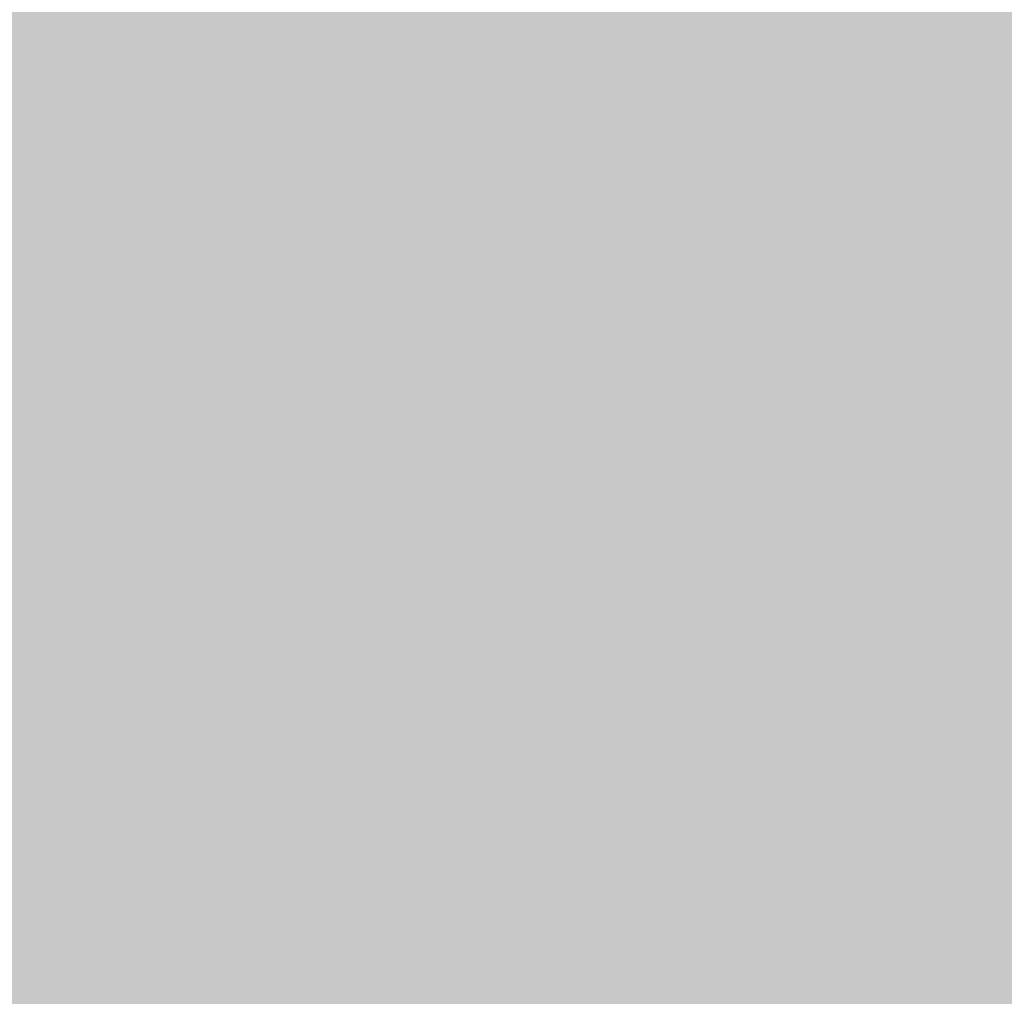
# Model space of a CAD drawing. Units: inches. Extents: x 2083 to 3317, y 1141 to 2115.
# Tile 162 of 256: x 3126.958245 to 3126.959398, y 1263.262504 to 1263.263648. Entities that reach past the tile are written whole.
import ezdxf

# ---------------------------------------------------------------- set-up
doc = ezdxf.new("R2010")
doc.units = ezdxf.units.IN
doc.layers.add('A-WALL-PATT', color=251, linetype='Continuous', lineweight=13, true_color=0x636466)

msp = doc.modelspace()

# ---------------------------------------------------------------- hatches: boundary and pattern name
at = {"layer": 'A-WALL-PATT'}
h = msp.add_hatch(color=256, dxfattribs=at)
h.dxf.hatch_style = 1
h.paths.add_polyline_path([(3126.9597832, 2020.7613601), (2748.9597832, 2020.7613601), (2604.9597832, 2020.7613601), (2226.9597832, 2020.7613601), (2226.9597832, 1702.7613601), (2466.9597832, 1702.7613601), (2466.9597832, 1582.7613601), (2418.9597832, 1582.7613601), (2418.9597832, 1477.7613601), (2226.9597832, 1477.7613601), (2226.9597832, 1263.2613601), (2544.9597832, 1263.2613601), (2544.9597832, 1411.7613601), (2604.9597832, 1411.7613601), (2685.9597832, 1411.7613601), (2685.9597832, 1420.7613601), (2604.9597832, 1420.7613601), (2604.9597832, 1573.7613601), (2604.9597832, 1702.7613601), (2604.9597832, 2011.7613601), (2748.9597832, 2011.7613601), (2748.9597832, 1702.7613601), (2862.9597832, 1702.7613601), (2862.9597832, 1621.7613601), (2871.9597832, 1621.7613601), (2871.9597832, 1702.7613601), (2883.9597832, 1702.7613601), (2883.9597832, 1706.9394595, -0.026459), (2883.9597832, 1711.7613601), (2757.9597832, 1711.7613601), (2757.9597832, 1807.7613601), (2787.9597832, 1807.7613601), (2787.9597832, 1812.2613601), (2757.9597832, 1812.2613601), (2757.9597832, 2011.7613601), (2877.9597832, 2011.7613601), (2877.9597832, 1812.2613601), (2847.9597832, 1812.2613601), (2847.9597832, 1807.7613601), (2889.8357425, 1807.7613601), (2889.8357425, 1812.2613601), (2882.4597832, 1812.2613601), (2882.4597832, 2011.7613601), (3117.9597832, 2011.7613601), (3117.9597832, 1812.2613601), (2937.8357425, 1812.2613601), (2937.8357425, 1807.7613601), (2995.7097832, 1807.7613601), (2995.7097832, 1796.1176655), (3000.2097832, 1796.1176655), (3000.2097832, 1807.7613601), (3117.9597832, 1807.7613601), (3117.9597832, 1711.7613601), (3000.2097832, 1711.7613601), (3000.2097832, 1760.1176655), (2998.5727047, 1760.1176655, -0.020711), (2995.7097832, 1760.1176655), (2995.7097832, 1711.7613601), (2931.9597832, 1711.7613601), (2931.9597832, 1702.7613601), (3126.9597832, 1702.7613601)])
h.paths.add_polyline_path([(2471.4597832, 2011.7613601), (2471.4597832, 1810.0113601), (2462.7169357, 1810.0113601), (2462.7169357, 1805.5113601), (2505.9597832, 1805.5113601), (2505.9597832, 1810.0113601), (2475.9597832, 1810.0113601), (2475.9597832, 2011.7613601), (2595.9597832, 2011.7613601), (2595.9597832, 1810.0113601), (2565.9597832, 1810.0113601), (2565.9597832, 1805.5113601), (2595.9597832, 1805.5113601), (2595.9597832, 1711.7613601), (2235.9597832, 1711.7613601), (2235.9597832, 1805.5113601), (2353.7097832, 1805.5113601), (2353.7097832, 1796.0541624), (2358.2097832, 1796.0541624), (2358.2097832, 1805.5113601), (2414.7169357, 1805.5113601), (2414.7169357, 1810.0113601), (2235.9597832, 1810.0113601), (2235.9597832, 2011.7613601)], flags=16)
h.paths.add_polyline_path([(2270.2047343, 1994.6100082), (2270.2047343, 1970.6100082), (2246.2047343, 1970.6100082), (2246.2047343, 1994.6100082)], flags=0)
edge = h.paths.add_edge_path(flags=0)
edge.add_ellipse((2332.027391, 1899.7981761), major_axis=(-3.0429938, 3.0429938), ratio=0.16825245, start_angle=-161.3321656, end_angle=-156.3071136, ccw=False)
edge.add_ellipse((2333.0820373, 1898.7435297), major_axis=(-1.0546463, 1.0546463), ratio=0.453532097, start_angle=-123.371019, end_angle=-94.1591066)
edge = h.paths.add_edge_path(flags=0)
edge.add_ellipse((2332.027391, 1968.8762897), major_axis=(3.0429938, 3.0429938), ratio=0.16825245, start_angle=18.6678344, end_angle=23.6928864)
edge.add_spline(control_points=[(2332.9255964, 1970.6911045), (2332.2267681, 1970.3360997), (2330.8937087, 1969.6589054), (2328.4130803, 1970.9321376), (2327.2039345, 1967.7487119), (2324.7095965, 1969.9555886), (2322.5328223, 1967.012354), (2320.0128462, 1971.2958124), (2317.6803077, 1968.1578449), (2316.0405263, 1967.1020468), (2315.4269045, 1966.8096022)], knot_values=[0, 0, 0, 0, 2.267059, 4.324559, 6.685584, 8.878641, 11.121502, 14.300359, 17.755284, 19.732645, 19.732645, 19.732645, 19.732645], degree=3, periodic=0)
edge.add_ellipse((2332.027391, 1968.8762897), major_axis=(3.0429938, 3.0429938), ratio=0.16825245, start_angle=18.6678344, end_angle=23.6928864, ccw=False)
edge.add_ellipse((2333.0820373, 1969.930936), major_axis=(1.0546463, 1.0546463), ratio=0.453532097, start_angle=56.628981, end_angle=85.8408934, ccw=False)
edge = h.paths.add_edge_path(flags=0)
edge.add_spline(control_points=[(2296.4282874, 1967.9879081), (2293.6278045, 1965.3363137), (2287.7036238, 1959.727094), (2299.7438601, 1949.9956993), (2294.5325909, 1935.6685275), (2290.5732281, 1920.6035119), (2293.3941244, 1909.9736911), (2296.1854073, 1904.9665431)], knot_values=[0.099185, 0.099185, 0.099185, 0.099185, 0.345301, 0.619822, 0.982653, 1.386093, 1.810555, 1.810555, 1.810555, 1.810555], degree=3, periodic=0)
edge.add_spline(control_points=[(2296.1854073, 1904.9665431), (2297.3835817, 1902.6193002), (2298.0009694, 1901.9493116), (2298.5529698, 1901.4681549)], knot_values=[0.006246, 0.006246, 0.006246, 0.006246, 0.055476, 0.055476, 0.055476, 0.055476], degree=3, periodic=0)
edge.add_spline(control_points=[(2298.5529698, 1901.4681549), (2297.2586121, 1900.9232238), (2295.2252939, 1900.2321257), (2293.0602287, 1900.6142053), (2292.1014227, 1900.788415), (2292.0895776, 1900.790568)], knot_values=[0.312835, 0.312835, 0.312835, 0.312835, 0.40178, 0.474987, 0.475903, 0.475903, 0.475903, 0.475903], degree=3, periodic=0)
edge.add_arc((2292.7936464, 1904.6641088), 3.9370079, 215.4208969, 259.6981795, ccw=False)
edge.add_spline(control_points=[(2289.5853139, 1902.3823039), (2289.4766524, 1902.5350874), (2289.3684805, 1902.6880353), (2289.2608648, 1902.8411699)], knot_values=[0.102872, 0.102872, 0.102872, 0.102872, 0.116896, 0.116896, 0.116896, 0.116896], degree=3, periodic=0)
edge.add_spline(control_points=[(2289.2608648, 1902.8411699), (2288.6866042, 1902.5501922), (2287.6400477, 1902.0199025), (2285.8813368, 1901.8739536), (2283.8529717, 1901.5043521), (2281.7199871, 1899.7105375), (2278.4669913, 1899.492942), (2276.1571361, 1901.8832022), (2272.2589526, 1899.8040711), (2267.7776054, 1901.8431828), (2262.2438819, 1900.1840326), (2257.414927, 1901.7820606), (2254.318374, 1900.7261196), (2253.1782849, 1900.3373431)], knot_values=[0, 0, 0, 0, 1.907977, 3.477176, 5.261074, 7.972851, 11.680248, 13.717921, 16.939592, 22.789562, 27.502503, 33.595215, 37.145618, 37.145618, 37.145618, 37.145618], degree=3, periodic=0)
edge.add_line((2253.1782849, 1900.3373431), (2250.2442397, 1902.8411699))
edge.add_line((2250.2442397, 1902.8411699), (2250.2442397, 1965.8332959))
edge.add_line((2250.2442397, 1965.8332959), (2253.1782849, 1968.3371226))
edge.add_spline(control_points=[(2253.1782849, 1968.3371226), (2254.318374, 1967.9483462), (2257.414927, 1966.8924051), (2262.2438819, 1968.4904332), (2267.7776054, 1966.8312829), (2271.5267301, 1968.5372172), (2273.8759143, 1967.8282895), (2274.2067012, 1967.7276424)], knot_values=[0, 0, 0, 0, 0.09018, 0.244935, 0.364644, 0.513233, 0.537855, 0.537855, 0.537855, 0.537855], degree=3, periodic=0)
edge.add_arc((2274.3528869, 1963.7933495), 3.9370079, 72.0511336, 92.1279492, ccw=False)
edge.add_arc((2281.2969331, 1985.2300027), 18.5962982, 252.05113361, 288.56572166)
edge.add_arc((2292.3167172, 1956.0288805), 12.6460805, 71.02678788, 113.77821843, ccw=False)
edge = h.paths.add_edge_path(flags=0)
edge.add_spline(control_points=[(2274.8994147, 1951.8561946), (2275.066156, 1951.6165924), (2275.2326866, 1951.3765878), (2275.3979871, 1951.1358545)], knot_values=[1.409916, 1.409916, 1.409916, 1.409916, 1.43159, 1.43159, 1.43159, 1.43159], degree=3, periodic=0)
edge.add_spline(control_points=[(2275.3979871, 1951.1358545), (2275.7921055, 1950.5618854), (2276.1792311, 1949.9837745), (2276.5455462, 1949.3971029)], knot_values=[1.358238, 1.358238, 1.358238, 1.358238, 1.409916, 1.409916, 1.409916, 1.409916], degree=3, periodic=0)
edge.add_line((2276.5455462, 1949.3971029), (2277.437289, 1947.8621847))
edge.add_spline(control_points=[(2277.437289, 1947.8621847), (2276.3038341, 1945.6731147), (2274.6396979, 1942.4268817), (2274.631615, 1938.0938998), (2272.7991237, 1930.8515498), (2274.3564261, 1943.8970461), (2275.9476814, 1947.9233558), (2276.5455462, 1949.3971029)], knot_values=[0.005632, 0.005632, 0.005632, 0.005632, 0.186014, 0.266002, 0.357087, 0.59639, 0.739732, 0.739732, 0.739732, 0.739732], degree=3, periodic=0)
edge.add_spline(control_points=[(2276.5455462, 1949.3971029), (2276.1792311, 1949.9837745), (2275.7921055, 1950.5618854), (2275.3979871, 1951.1358545)], knot_values=[1.358238, 1.358238, 1.358238, 1.358238, 1.409916, 1.409916, 1.409916, 1.409916], degree=3, periodic=0)
edge.add_spline(control_points=[(2275.3979871, 1951.1358545), (2274.9425002, 1950.0804523), (2274.2077604, 1948.0252718), (2273.9346018, 1944.8514774), (2272.4685341, 1937.6274891), (2273.4662155, 1945.6964663), (2274.7006154, 1951.0594725), (2274.8994147, 1951.8561946)], knot_values=[0.104364, 0.104364, 0.104364, 0.104364, 0.189636, 0.269624, 0.36071, 0.600013, 0.644622, 0.644622, 0.644622, 0.644622], degree=3, periodic=0)
h.paths.add_polyline_path([(2269.1675139, 1963.1275729, -0.357527), (2268.170633, 1960.9763695, -0.092561), (2268.170633, 1939.4363249, -0.357527), (2269.1675139, 1937.2851215, -0.357527), (2267.0163105, 1938.2820024, -0.164785), (2254.6855813, 1938.2820024, -0.357527), (2252.5343779, 1937.2851215, -0.357527), (2253.5312587, 1939.4363249, -0.092561), (2253.5312587, 1960.9763695, -0.357527), (2252.5343779, 1963.1275729, -0.357527), (2254.6855813, 1962.130692, -0.164785), (2267.0163105, 1962.130692, -0.357527)], flags=0)
h.paths.add_polyline_path([(2248.8740679, 1967.8017998), (2248.8740679, 1957.0277095), (2249.4577833, 1957.0277095), (2249.4577833, 1911.6467562), (2248.8740679, 1911.6467562), (2248.8740679, 1900.8726659), (2246.5118632, 1900.8726659, 0.197327), (2244.1496584, 1902.4568734), (2244.1496584, 1966.2175923, 0.197327), (2246.5118632, 1967.8017998)], flags=0)
h.paths.add_polyline_path([(2269.1675139, 1931.3893442, -0.357527), (2268.170633, 1929.2381408, -0.092561), (2268.170633, 1907.6980962, -0.357527), (2269.1675139, 1905.5468928, -0.357527), (2267.0163105, 1906.5437737, -0.164785), (2254.6855813, 1906.5437737, -0.357527), (2252.5343779, 1905.5468928, -0.357527), (2253.5312587, 1907.6980962, -0.092561), (2253.5312587, 1929.2381408, -0.357527), (2252.5343779, 1931.3893442, -0.357527), (2254.6855813, 1930.3924634, -0.164785), (2267.0163105, 1930.3924634, -0.357527)], flags=0)
edge = h.paths.add_edge_path(flags=0)
edge.add_spline(control_points=[(2276.1968578, 1906.7237016), (2276.1681442, 1909.0289278), (2276.1140492, 1913.371852), (2270.5984171, 1924.9249783), (2273.9051746, 1919.0127787), (2275.9217115, 1916.2620626), (2275.4745699, 1912.4021495), (2277.2578735, 1910.3806206), (2276.6960436, 1908.2250358), (2276.6462176, 1906.8130226), (2276.6178249, 1906.0084068)], knot_values=[0, 0, 0, 0, 8.61026, 16.221274, 18.843057, 23.804898, 27.440828, 29.356102, 31.203478, 33.650687, 33.650687, 33.650687, 33.650687], degree=3, periodic=0)
edge.add_spline(control_points=[(2276.6178249, 1906.0084068), (2276.6233131, 1905.6241436), (2276.4977381, 1904.6286608), (2275.4417789, 1903.8547251), (2274.9373144, 1903.0804497), (2274.8590804, 1902.8411699)], knot_values=[0.156488, 0.156488, 0.156488, 0.156488, 0.184398, 0.231376, 0.250598, 0.250598, 0.250598, 0.250598], degree=3, periodic=0)
edge.add_line((2274.8590804, 1902.8411699), (2276.50598, 1902.8411699))
edge.add_spline(control_points=[(2276.50598, 1902.8411699), (2276.7883084, 1903.0849395), (2277.6650711, 1904.1251958), (2278.2495378, 1904.340738), (2277.6538719, 1908.5273866), (2278.15567, 1906.2278078), (2278.100464, 1905.2859484), (2278.8466748, 1904.0690054), (2277.8567853, 1903.4149482), (2277.8741909, 1902.9910497), (2277.9035616, 1902.8411699)], knot_values=[0.059574, 0.059574, 0.059574, 0.059574, 0.080753, 0.103741, 0.16972, 0.176036, 0.207137, 0.240474, 0.262341, 0.27366, 0.27366, 0.27366, 0.27366], degree=3, periodic=0)
edge.add_line((2277.9035616, 1902.8411699), (2280.0298255, 1902.8411699))
edge.add_spline(control_points=[(2280.0298255, 1902.8411699), (2279.8882214, 1903.088398), (2279.4992571, 1903.9815512), (2280.1522839, 1905.9393491), (2278.103615, 1909.6577572), (2279.7623946, 1907.185285), (2280.3279002, 1904.8748608), (2280.4851086, 1903.4895904), (2281.4632687, 1903.2494323), (2281.7583431, 1902.9364967), (2281.8340361, 1902.8411699)], knot_values=[0.013856, 0.013856, 0.013856, 0.013856, 0.034874, 0.088867, 0.107879, 0.126738, 0.158714, 0.193757, 0.217487, 0.226722, 0.226722, 0.226722, 0.226722], degree=3, periodic=0)
edge.add_spline(control_points=[(2281.8340361, 1902.8411699), (2281.7875348, 1902.8267029), (2281.6470224, 1902.7829881), (2281.3955272, 1902.85949), (2281.088077, 1902.9852418), (2280.7206826, 1903.060902), (2280.3334513, 1903.0257257), (2280.1247668, 1902.898879), (2280.0298255, 1902.8411699)], knot_values=[0, 0, 0, 0, 0.14413, 0.435517, 0.749276, 1.153046, 1.548371, 1.878348, 1.878348, 1.878348, 1.878348], degree=3, periodic=0)
edge.add_line((2280.0298255, 1902.8411699), (2277.9035616, 1902.8411699))
edge.add_spline(control_points=[(2277.9035616, 1902.8411699), (2277.892855, 1902.7958553), (2277.865396, 1902.6796374), (2277.6074793, 1902.6874828), (2277.2740503, 1902.8006999), (2276.8379209, 1902.6197745), (2276.5838074, 1902.7892611), (2276.50598, 1902.8411699)], knot_values=[0, 0, 0, 0, 0.127189, 0.326199, 0.628009, 1.24357, 1.515331, 1.515331, 1.515331, 1.515331], degree=3, periodic=0)
edge.add_line((2276.50598, 1902.8411699), (2274.8590804, 1902.8411699))
edge.add_spline(control_points=[(2274.8590804, 1902.8411699), (2274.8144367, 1902.8985868), (2274.7251297, 1903.013446), (2274.4934765, 1903.1189684), (2274.2442854, 1902.9605386), (2273.9371207, 1903.1849416), (2273.6140395, 1902.9831428), (2273.4083164, 1902.8830449), (2273.322254, 1902.8411699)], knot_values=[0, 0, 0, 0, 0.21843, 0.436957, 0.687977, 0.990379, 1.398396, 1.69185, 1.69185, 1.69185, 1.69185], degree=3, periodic=0)
edge.add_spline(control_points=[(2273.322254, 1902.8411699), (2273.6167403, 1903.445692), (2274.2739977, 1904.5382529), (2276.0272387, 1904.5737017), (2276.2069634, 1906.5836372), (2276.1968578, 1906.7237016)], knot_values=[0.012227, 0.012227, 0.012227, 0.012227, 0.059472, 0.106218, 0.134458, 0.134458, 0.134458, 0.134458], degree=3, periodic=0)
h.paths.add_polyline_path([(2270.7760538, 1897.7898284), (2270.7760538, 1873.7898284), (2246.7760538, 1873.7898284), (2246.7760538, 1897.7898284)], flags=0)
h.paths.add_polyline_path([(2353.7097832, 1760.0050593), (2353.7097832, 1760.0541624), (2358.2097832, 1760.0541624, -0.033729)], flags=0)
h.paths.add_polyline_path([(2321.8191188, 1737.5291862), (2341.9953271, 1737.5291862, -0.414214), (2343.2032727, 1736.3212406), (2343.2032727, 1721.0205964, -0.414214), (2341.9953271, 1719.8126508), (2321.8191188, 1719.8126508, -0.414214), (2320.6111732, 1721.0205964), (2320.6111732, 1736.3212406, -0.414214)], flags=0)
h.paths.add_polyline_path([(2324.2350099, 1736.3212406), (2339.5794359, 1736.3212406, -0.414214), (2341.9953271, 1733.9053494), (2341.9953271, 1725.4497302, -0.414214), (2339.5794359, 1723.033839), (2333.6805885, 1723.033839), (2333.8453172, 1722.0454666, -0.870646), (2335.4253988, 1721.8258934, -0.767327), (2333.922694, 1721.4232449), (2331.2910241, 1721.4232449, -0.767327), (2329.7883193, 1721.8258934, -0.870646), (2331.3684009, 1722.0454666), (2331.5331296, 1723.033839), (2324.2350099, 1723.033839, -0.414214), (2321.8191188, 1725.4497302), (2321.8191188, 1733.9053494, -0.414214)], flags=0)
h.paths.add_polyline_path([(2570.4837892, 1928.6154443), (2589.6837892, 1928.6154443), (2590.1688286, 1928.6154443), (2590.1688286, 1904.9933971), (2570.4837892, 1904.9933971)], flags=0)
h.paths.add_polyline_path([(2574.4473242, 1927.2638215, -1), (2572.8288357, 1927.2638215, -1)], flags=0)
h.paths.add_polyline_path([(2573.0898665, 1926.9408768), (2573.925032, 1927.7760423), (2574.1477428, 1927.5533315), (2573.3125773, 1926.718166)], flags=0)
h.paths.add_polyline_path([(2578.7790648, 1919.7296175, -1), (2571.5916632, 1919.7296175, -1)], flags=0)
h.paths.add_polyline_path([(2578.385364, 1919.7296175, -1), (2571.985364, 1919.7296175, -1)], flags=0)
h.paths.add_polyline_path([(2331.5957638, 1729.4762156, -1), (2333.6179542, 1729.4762156, -1)], flags=0)
h.paths.add_polyline_path([(2578.0342282, 1927.2638215, -1), (2576.4157396, 1927.2638215, -1)], flags=0)
h.paths.add_polyline_path([(2576.6888513, 1927.5310886), (2576.9115621, 1927.7537993), (2577.7467276, 1926.9186339), (2577.5240168, 1926.6959231)], flags=0)
h.paths.add_polyline_path([(2578.1390648, 1909.8595388, -1), (2572.2316632, 1909.8595388, -1)], flags=0)
h.paths.add_polyline_path([(2577.745364, 1909.8595388, -1), (2572.625364, 1909.8595388, -1)], flags=0)
h.paths.add_polyline_path([(2583.7977179, 1927.2638215, -1), (2582.1792294, 1927.2638215, -1)], flags=0)
h.paths.add_polyline_path([(2582.7186487, 1927.7537993), (2583.5538142, 1926.9186339), (2583.3311034, 1926.6959231), (2582.4959379, 1927.5310886)], flags=0)
h.paths.add_polyline_path([(2582.4959379, 1927.5310886), (2582.7186487, 1927.7537993), (2583.5538142, 1926.9186339), (2583.3311034, 1926.6959231)], flags=0)
h.paths.add_polyline_path([(2587.7390648, 1920.5296175, -1), (2581.8316632, 1920.5296175, -1)], flags=0)
h.paths.add_polyline_path([(2587.345364, 1920.5296175, -1), (2582.225364, 1920.5296175, -1)], flags=0)
h.paths.add_polyline_path([(2587.3846219, 1927.2638215, -1), (2585.7661333, 1927.2638215, -1)], flags=0)
h.paths.add_polyline_path([(2586.0819925, 1926.9802469), (2586.917158, 1927.8154124), (2587.1398688, 1927.5927016), (2586.3047033, 1926.7575361)], flags=0)
h.paths.add_polyline_path([(2588.3790648, 1910.6595388, -1), (2581.1916632, 1910.6595388, -1)], flags=0)
h.paths.add_polyline_path([(2587.985364, 1910.6595388, -1), (2581.585364, 1910.6595388, -1)], flags=0)
h.paths.add_polyline_path([(2417.1677288, 1729.4778955), (2437.3439372, 1729.4778955, -0.414214), (2438.5518828, 1728.2699499), (2438.5518828, 1712.9693057, -0.414214), (2437.3439372, 1711.7613601), (2417.1677288, 1711.7613601, -0.414214), (2415.9597832, 1712.9693057), (2415.9597832, 1728.2699499, -0.414214)], flags=0)
h.paths.add_polyline_path([(2419.58362, 1728.2699499), (2434.928046, 1728.2699499, -0.414214), (2437.3439372, 1725.8540587), (2437.3439372, 1717.3984395, -0.414214), (2434.928046, 1714.9825483), (2429.0291985, 1714.9825483), (2429.1939273, 1713.9941758, -0.870646), (2430.7740089, 1713.7746027, -0.767327), (2429.2713041, 1713.3719542), (2426.6396342, 1713.3719542, -0.767327), (2425.1369294, 1713.7746027, -0.870646), (2426.717011, 1713.9941758), (2426.8817397, 1714.9825483), (2419.58362, 1714.9825483, -0.414214), (2417.1677288, 1717.3984395), (2417.1677288, 1725.8540587, -0.414214)], flags=0)
h.paths.add_polyline_path([(2419.58362, 1728.2699499), (2434.928046, 1728.2699499, -0.414214), (2437.3439372, 1725.8540587), (2437.3439372, 1717.3984395, -0.414214), (2434.928046, 1714.9825483), (2429.0291985, 1714.9825483), (2428.3581177, 1719.0090337), (2427.5528206, 1719.0090337), (2426.8817397, 1714.9825483), (2419.58362, 1714.9825483, -0.414214), (2417.1677288, 1717.3984395), (2417.1677288, 1725.8540587, -0.414214)], flags=0)
h.paths.add_polyline_path([(2426.9443739, 1721.4249248, -1), (2428.9665643, 1721.4249248, -1)], flags=0)
h.paths.add_polyline_path([(2475.9597832, 1702.7613601), (2595.9597832, 1702.7613601), (2595.9597832, 1582.7613601), (2475.9597832, 1582.7613601)], flags=16)
h.paths.add_polyline_path([(2427.9597832, 1573.7613601), (2595.9597832, 1573.7613601), (2595.9597832, 1468.7613601), (2595.9597832, 1420.7613601), (2384.4597832, 1420.7613601), (2384.4597832, 1468.7613601), (2427.9597832, 1468.7613601)], flags=16)
h.paths.add_polyline_path([(2379.9597832, 1468.7613601), (2379.9597832, 1420.7613601), (2235.9597832, 1420.7613601), (2235.9597832, 1468.7613601)], flags=16)
h.paths.add_polyline_path([(2317.8159962, 1466.695767), (2337.9922045, 1466.695767, -0.414214), (2339.2001501, 1465.4878214), (2339.2001501, 1450.1871771, -0.414214), (2337.9922045, 1448.9792315), (2317.8159962, 1448.9792315, -0.414214), (2316.6080506, 1450.1871771), (2316.6080506, 1465.4878214, -0.414214)], flags=0)
h.paths.add_polyline_path([(2320.2318874, 1465.4878214), (2335.5763133, 1465.4878214, -0.414214), (2337.9922045, 1463.0719302), (2337.9922045, 1454.616311, -0.414214), (2335.5763133, 1452.2004198), (2329.6774659, 1452.2004198), (2329.8421946, 1451.2120473, -0.870646), (2331.4222762, 1450.9924742, -0.767327), (2329.9195714, 1450.5898257), (2327.2879015, 1450.5898257, -0.767327), (2325.7851967, 1450.9924742, -0.870646), (2327.3652783, 1451.2120473), (2327.530007, 1452.2004198), (2320.2318874, 1452.2004198, -0.414214), (2317.8159962, 1454.616311), (2317.8159962, 1463.0719302, -0.414214)], flags=0)
h.paths.add_polyline_path([(2320.2318874, 1465.4878214), (2335.5763133, 1465.4878214, -0.414214), (2337.9922045, 1463.0719302), (2337.9922045, 1454.616311, -0.414214), (2335.5763133, 1452.2004198), (2329.6774659, 1452.2004198), (2329.006385, 1456.2269051), (2328.2010879, 1456.2269051), (2327.530007, 1452.2004198), (2320.2318874, 1452.2004198, -0.414214), (2317.8159962, 1454.616311), (2317.8159962, 1463.0719302, -0.414214)], flags=0)
h.paths.add_polyline_path([(2327.5926413, 1458.6427963, -1), (2329.6148317, 1458.6427963, -1)], flags=0)
h.paths.add_polyline_path([(2244.4117436, 1433.3404531), (2241.9209449, 1433.3404531, -0.414214), (2240.0178562, 1435.2435418), (2240.0178562, 1440.9528078, -0.414211), (2241.920925, 1442.8558965), (2244.4117436, 1442.8558965, -1.976472)], flags=0)
h.paths.add_polyline_path([(2245.3568884, 1434.3975358, -0.414214), (2245.3568884, 1441.7988138, -2.144098)], flags=0)
h.paths.add_polyline_path([(2535.9597832, 1416.2613601), (2535.9597832, 1272.2613601), (2235.9597832, 1272.2613601), (2235.9597832, 1416.2613601)], flags=16)
h.paths.add_polyline_path([(2260.1195614, 1384.2928413), (2260.1195614, 1362.0386487), (2237.8653688, 1362.0386487), (2237.8653688, 1384.2928413)], flags=0)
edge = h.paths.add_edge_path(flags=0)
edge.add_line((2318.2518466, 1362.0932983), (2318.1457968, 1362.0009726))
edge.add_ellipse((2317.4451158, 1360.4310442), major_axis=(2.8216404, 2.8216404), ratio=0.16825245, start_angle=18.6678344, end_angle=20.9481273, ccw=False)
edge.add_ellipse((2318.4230451, 1361.4089735), major_axis=(0.9779293, 0.9779293), ratio=0.453532097, start_angle=56.628981, end_angle=70.2262012, ccw=False)
edge = h.paths.add_edge_path(flags=0)
edge.add_line((2319.1073699, 1295.5710784), (2319.0150442, 1295.6771282))
edge.add_ellipse((2317.4451158, 1296.3778091), major_axis=(-2.8216404, 2.8216404), ratio=0.16825245, start_angle=-161.3321656, end_angle=-159.0518727, ccw=False)
edge.add_ellipse((2318.4230451, 1295.3998798), major_axis=(-0.9779293, 0.9779293), ratio=0.453532097, start_angle=-123.371019, end_angle=-109.7737988)
edge = h.paths.add_edge_path(flags=0)
edge.add_spline(control_points=[(2284.2103489, 1301.1702189), (2284.5806878, 1300.444719), (2284.8911891, 1299.8920243), (2285.159553, 1299.4610182)], knot_values=[0.039066, 0.039066, 0.039066, 0.039066, 0.055476, 0.055476, 0.055476, 0.055476], degree=3, periodic=0)
edge.add_line((2285.159553, 1299.4610182), (2284.2103489, 1301.1702189))
edge = h.paths.add_edge_path(flags=0)
edge.add_line((2280.4124579, 1297.2980125), (2283.3699905, 1297.0361216))
edge.add_line((2283.3699905, 1297.0361216), (2286.4056902, 1297.9263104))
edge.add_spline(control_points=[(2286.4056902, 1297.9263104), (2285.305487, 1297.4631193), (2284.3447774, 1297.1291508), (2283.3699905, 1297.0361216)], knot_values=[0.394369, 0.394369, 0.394369, 0.394369, 0.475903, 0.475903, 0.475903, 0.475903], degree=3, periodic=0)
edge.add_spline(control_points=[(2283.3699905, 1297.0361216), (2283.2813895, 1297.027666), (2282.316289, 1296.9573356), (2281.3125019, 1297.1344787), (2280.4234414, 1297.2960161), (2280.4124579, 1297.2980125)], knot_values=[0.312835, 0.312835, 0.312835, 0.312835, 0.320246, 0.393453, 0.394369, 0.394369, 0.394369, 0.394369], degree=3, periodic=0)
edge = h.paths.add_edge_path(flags=0)
edge.add_line((2284.4355615, 1359.6072854), (2280.4462909, 1355.328047))
edge.add_line((2280.4462909, 1355.328047), (2279.5799868, 1351.0177544))
edge.add_line((2279.5799868, 1351.0177544), (2282.4129737, 1346.5804327))
edge.add_spline(control_points=[(2282.4129737, 1346.5804327), (2283.1533308, 1345.5892358), (2284.2528957, 1344.0288973), (2284.801037, 1342.3871671), (2284.9351625, 1341.8055443)], knot_values=[1.240098, 1.240098, 1.240098, 1.240098, 1.332892, 1.382712, 1.382712, 1.382712, 1.382712], degree=3, periodic=0)
edge.add_spline(control_points=[(2284.9351625, 1341.8055443), (2285.3191079, 1340.1406002), (2285.2330291, 1338.4092041), (2284.9099384, 1336.6541222)], knot_values=[1.097484, 1.097484, 1.097484, 1.097484, 1.240098, 1.240098, 1.240098, 1.240098], degree=3, periodic=0)
edge.add_spline(control_points=[(2284.9099384, 1336.6541222), (2284.5868478, 1334.8990403), (2284.0267453, 1333.1202725), (2283.4626437, 1331.3605849)], knot_values=[0.95487, 0.95487, 0.95487, 0.95487, 1.097484, 1.097484, 1.097484, 1.097484], degree=3, periodic=0)
edge.add_line((2283.4626437, 1331.3605849), (2281.8903759, 1326.153357))
edge.add_line((2281.8903759, 1326.153357), (2280.7562592, 1321.0560888))
edge.add_line((2280.7562592, 1321.0560888), (2280.2992048, 1316.0019772))
edge.add_line((2280.2992048, 1316.0019772), (2280.7159327, 1310.9500678))
edge.add_line((2280.7159327, 1310.9500678), (2282.0280939, 1305.9721367))
edge.add_line((2282.0280939, 1305.9721367), (2284.2103489, 1301.1702189))
edge.add_spline(control_points=[(2284.2103489, 1301.1702189), (2283.3407305, 1302.7301854), (2282.6119044, 1304.3364933), (2282.0280939, 1305.9721367)], knot_values=[0.099185, 0.099185, 0.099185, 0.099185, 0.241799, 0.241799, 0.241799, 0.241799], degree=3, periodic=0)
edge.add_spline(control_points=[(2282.0280939, 1305.9721367), (2281.4442835, 1307.6077801), (2281.0054886, 1309.2727591), (2280.7159327, 1310.9500678)], knot_values=[0.241799, 0.241799, 0.241799, 0.241799, 0.384413, 0.384413, 0.384413, 0.384413], degree=3, periodic=0)
edge.add_spline(control_points=[(2280.7159327, 1310.9500678), (2280.4332411, 1312.5876134), (2280.2893863, 1314.2769594), (2280.2988938, 1315.9620324), (2280.2992048, 1316.0019772)], knot_values=[0.384413, 0.384413, 0.384413, 0.384413, 0.523647, 0.527028, 0.527028, 0.527028, 0.527028], degree=3, periodic=0)
edge.add_spline(control_points=[(2280.2992048, 1316.0019772), (2280.3123257, 1317.6869552), (2280.4778706, 1319.3679256), (2280.7562592, 1321.0560888)], knot_values=[0.527028, 0.527028, 0.527028, 0.527028, 0.669642, 0.669642, 0.669642, 0.669642], degree=3, periodic=0)
edge.add_spline(control_points=[(2280.7562592, 1321.0560888), (2281.0346478, 1322.7442519), (2281.4258801, 1324.4396079), (2281.8903759, 1326.153357)], knot_values=[0.669642, 0.669642, 0.669642, 0.669642, 0.812256, 0.812256, 0.812256, 0.812256], degree=3, periodic=0)
edge.add_spline(control_points=[(2281.8903759, 1326.153357), (2282.2643834, 1327.5332507), (2282.7878702, 1329.2618097), (2283.352751, 1331.0177803), (2283.4626437, 1331.3605849)], knot_values=[0.812256, 0.812256, 0.812256, 0.812256, 0.927087, 0.95487, 0.95487, 0.95487, 0.95487], degree=3, periodic=0)
edge.add_line((2283.4626437, 1331.3605849), (2284.9099384, 1336.6541222))
edge.add_line((2284.9099384, 1336.6541222), (2284.9351625, 1341.8055443))
edge.add_line((2284.9351625, 1341.8055443), (2282.4129737, 1346.5804327))
edge.add_spline(control_points=[(2282.4129737, 1346.5804327), (2281.2751273, 1348.1037918), (2280.0784467, 1349.5703178), (2279.5799868, 1351.0177544)], knot_values=[1.382712, 1.382712, 1.382712, 1.382712, 1.525326, 1.525326, 1.525326, 1.525326], degree=3, periodic=0)
edge.add_spline(control_points=[(2279.5799868, 1351.0177544), (2279.4432818, 1351.4147209), (2279.1363124, 1352.856922), (2279.7351897, 1354.2903851), (2280.4462909, 1355.328047)], knot_values=[1.525326, 1.525326, 1.525326, 1.525326, 1.564439, 1.667941, 1.667941, 1.667941, 1.667941], degree=3, periodic=0)
edge.add_spline(control_points=[(2280.4462909, 1355.328047), (2281.4261132, 1356.7578354), (2282.9308373, 1358.1825604), (2284.4355615, 1359.6072854)], knot_values=[1.667941, 1.667941, 1.667941, 1.667941, 1.810555, 1.810555, 1.810555, 1.810555], degree=3, periodic=0)
edge.add_arc((2280.6230749, 1348.518181), 11.7261796, 71.02678788, 113.77821843)
edge.add_arc((2270.4048917, 1375.5951559), 17.2435667, 252.05113361, 288.56572166, ccw=False)
edge.add_arc((2263.9659692, 1355.7178471), 3.6506221, 72.0511336, 92.1279492)
edge.add_arc((2263.9659692, 1355.7178471), 3.6506221, 92.1279492, 177.98513)
edge.add_spline(control_points=[(2260.3176041, 1355.8461989), (2260.2604169, 1354.2206683), (2260.551278, 1350.1865469), (2262.9993445, 1346.7662507), (2264.4727415, 1344.6490245)], knot_values=[1.43159, 1.43159, 1.43159, 1.43159, 1.564144, 1.770695, 1.770695, 1.770695, 1.770695], degree=3, periodic=0)
edge.add_line((2264.4727415, 1344.6490245), (2264.9355904, 1343.9825301))
edge.add_spline(control_points=[(2263.8010444, 1340.2481052), (2263.8432379, 1340.5140884), (2264.0672444, 1341.7564652), (2264.5126928, 1343.0024532), (2264.9350468, 1343.9810834)], knot_values=[0.53657, 0.53657, 0.53657, 0.53657, 0.559349, 0.644622, 0.644622, 0.644622, 0.644622], degree=3, periodic=0)
edge.add_spline(control_points=[(2264.9350468, 1343.9810834), (2265.1177715, 1343.7149747), (2265.2988751, 1343.4479058), (2265.4767562, 1343.1793646)], knot_values=[1.384077, 1.384077, 1.384077, 1.384077, 1.409916, 1.409916, 1.409916, 1.409916], degree=3, periodic=0)
edge.add_spline(control_points=[(2265.4767562, 1343.1793646), (2265.6546373, 1342.9108234), (2265.8292958, 1342.64081), (2265.9991301, 1342.368812)], knot_values=[1.358238, 1.358238, 1.358238, 1.358238, 1.384077, 1.384077, 1.384077, 1.384077], degree=3, periodic=0)
edge.add_line((2265.9991301, 1342.368812), (2266.8260057, 1340.9455468))
edge.add_spline(control_points=[(2266.8260057, 1340.9455468), (2268.894401, 1337.0896912), (2271.3981727, 1325.8430009), (2270.5161644, 1310.5685568), (2275.9193759, 1301.860609), (2277.7895113, 1299.1994495)], knot_values=[0.116896, 0.116896, 0.116896, 0.116896, 0.472987, 1.050969, 1.313793, 1.313793, 1.313793, 1.313793], degree=3, periodic=0)
edge.add_spline(control_points=[(2277.7895113, 1299.1994495), (2277.8394051, 1299.1284519), (2277.8894277, 1299.0574975), (2277.9395717, 1298.9865839)], knot_values=[0.109884, 0.109884, 0.109884, 0.109884, 0.116896, 0.116896, 0.116896, 0.116896], degree=3, periodic=0)
edge.add_line((2277.9395717, 1298.9865839), (2277.7888489, 1299.1991139))
edge.add_spline(control_points=[(2277.7888489, 1299.1991139), (2277.2565819, 1298.9294144), (2276.2863504, 1298.4379024), (2275.0393517, 1298.3344186), (2274.3833299, 1298.2388951), (2274.2152543, 1298.209338)], knot_values=[33.12187, 33.12187, 33.12187, 33.12187, 35.029056, 36.598255, 37.144827, 37.144827, 37.144827, 37.144827], degree=3, periodic=0)
edge.add_line((2274.2152543, 1298.209338), (2273.073147, 1297.8929607))
edge.add_spline(control_points=[(2273.073147, 1297.8929607), (2272.3229363, 1297.579784), (2271.0391507, 1296.5105078), (2269.2483948, 1296.2260622), (2268.4231004, 1296.3746543)], knot_values=[26.532584, 26.532584, 26.532584, 26.532584, 29.198919, 31.839101, 31.839101, 31.839101, 31.839101], degree=3, periodic=0)
edge.add_line((2268.4231004, 1296.3746543), (2263.8785014, 1297.4575338))
edge.add_spline(control_points=[(2263.8785014, 1297.4575338), (2263.5560769, 1297.3594345), (2261.8603064, 1296.8386943), (2260.2387805, 1297.2824073), (2258.9334543, 1297.5164611)], knot_values=[15.919551, 15.919551, 15.919551, 15.919551, 16.939592, 21.226067, 21.226067, 21.226067, 21.226067], degree=3, periodic=0)
edge.add_line((2258.9334543, 1297.5164611), (2254.0552332, 1297.3290098))
edge.add_spline(control_points=[(2254.0552332, 1297.3290098), (2253.7555255, 1297.295815), (2252.1136834, 1297.1651738), (2250.4618687, 1297.5442209), (2249.1296862, 1297.6678818)], knot_values=[5.306517, 5.306517, 5.306517, 5.306517, 6.276435, 10.613034, 10.613034, 10.613034, 10.613034], degree=3, periodic=0)
edge.add_line((2249.1296862, 1297.6678818), (2244.3316495, 1296.8777561))
edge.add_line((2244.3316495, 1296.8777561), (2241.6110326, 1299.1994495))
edge.add_line((2241.6110326, 1299.1994495), (2241.6110326, 1357.6094038))
edge.add_line((2241.6110326, 1357.6094038), (2244.3316495, 1359.9310973))
edge.add_line((2244.3316495, 1359.9310973), (2252.7288228, 1359.5426917))
edge.add_spline(control_points=[(2252.7288228, 1359.5426917), (2252.8709387, 1359.5464396), (2253.3057402, 1359.5481716), (2253.7398447, 1359.5142744), (2254.0317419, 1359.4824261)], knot_values=[0.233291, 0.233291, 0.233291, 0.233291, 0.244935, 0.268927, 0.268927, 0.268927, 0.268927], degree=3, periodic=0)
edge.add_line((2254.0317419, 1359.4824261), (2259.5871899, 1359.4163899))
edge.add_spline(control_points=[(2259.5871899, 1359.4163899), (2260.6770676, 1359.6285026), (2262.0731971, 1359.8970025), (2263.5236925, 1359.4592776), (2263.8304173, 1359.3659518)], knot_values=[0.422516, 0.422516, 0.422516, 0.422516, 0.513233, 0.537855, 0.537855, 0.537855, 0.537855], degree=3, periodic=0)
edge.add_arc((2263.9659692, 1355.7178471), 3.6506221, 72.0511336, 92.1279492, ccw=False)
edge.add_arc((2270.4048917, 1375.5951559), 17.2435667, 252.05113361, 288.56572166)
edge.add_arc((2280.6230749, 1348.518181), 11.7261796, 71.02678788, 113.77821843, ccw=False)
h.paths.add_polyline_path([(2240.3405298, 1359.4347149), (2240.3405298, 1349.4443532), (2240.8817846, 1349.4443532), (2240.8817846, 1307.3645001), (2240.3405298, 1307.3645001), (2240.3405298, 1297.3741385), (2238.1501565, 1297.3741385, 0.197327), (2235.9597832, 1298.8431076), (2235.9597832, 1357.9657458, 0.197327), (2238.1501565, 1359.4347149)], flags=0)
h.paths.add_polyline_path([(2259.1577904, 1355.1005005, -0.357527), (2258.2334246, 1353.1057799, -0.092561), (2258.2334246, 1333.1326007, -0.357527), (2259.1577904, 1331.1378801, -0.357527), (2257.1630698, 1332.0622458, -0.164785), (2245.7293022, 1332.0622458, -0.357527), (2243.7345816, 1331.1378801, -0.357527), (2244.6589474, 1333.1326007, -0.092561), (2244.6589474, 1353.1057799, -0.357527), (2243.7345816, 1355.1005005, -0.357527), (2245.7293022, 1354.1761347, -0.164785), (2257.1630698, 1354.1761347, -0.357527)], flags=0)
edge = h.paths.add_edge_path(flags=0)
edge.add_line((2265.9991301, 1342.368812), (2266.8260057, 1340.9455468))
edge.add_line((2266.8260057, 1340.9455468), (2265.3075567, 1337.8140664))
edge.add_line((2265.3075567, 1337.8140664), (2264.358232, 1334.6529388))
edge.add_line((2264.358232, 1334.6529388), (2264.2620123, 1333.7997046))
edge.add_spline(control_points=[(2264.2620123, 1333.7997046), (2264.2083565, 1333.187055), (2264.1620602, 1332.3655252), (2264.0071444, 1331.4139326), (2263.9690487, 1331.2018338)], knot_values=[0.464444, 0.464444, 0.464444, 0.464444, 0.516691, 0.531608, 0.531608, 0.531608, 0.531608], degree=3, periodic=0)
edge.add_spline(control_points=[(2263.9690487, 1331.2018338), (2263.7745349, 1330.1188727), (2263.4243703, 1328.7908386), (2263.2574202, 1328.5306516), (2263.2340282, 1328.5146115)], knot_values=[0.372682, 0.372682, 0.372682, 0.372682, 0.44885, 0.464444, 0.464444, 0.464444, 0.464444], degree=3, periodic=0)
edge.add_spline(control_points=[(2263.2340282, 1328.5146115), (2263.096382, 1328.4202271), (2263.1311696, 1329.3014765), (2263.2749528, 1330.6157493)], knot_values=[0.280919, 0.280919, 0.280919, 0.280919, 0.372682, 0.372682, 0.372682, 0.372682], degree=3, periodic=0)
edge.add_spline(control_points=[(2263.2749528, 1330.6157493), (2263.4187361, 1331.930022), (2263.6715151, 1333.677318), (2263.9698519, 1335.3150268)], knot_values=[0.189157, 0.189157, 0.189157, 0.189157, 0.280919, 0.280919, 0.280919, 0.280919], degree=3, periodic=0)
edge.add_spline(control_points=[(2263.9698519, 1335.3150268), (2264.1004958, 1336.0321917), (2264.4187827, 1337.6219113), (2264.7548476, 1338.8644304), (2264.9474193, 1339.4911244)], knot_values=[0.097394, 0.097394, 0.097394, 0.097394, 0.137578, 0.189157, 0.189157, 0.189157, 0.189157], degree=3, periodic=0)
edge.add_spline(control_points=[(2264.9474193, 1339.4911244), (2265.2900171, 1340.6060546), (2265.6442376, 1341.4939958), (2265.9991301, 1342.368812)], knot_values=[0.005632, 0.005632, 0.005632, 0.005632, 0.097394, 0.097394, 0.097394, 0.097394], degree=3, periodic=0)
h.paths.add_polyline_path([(2259.1577904, 1325.6709733, -0.357527), (2258.2334246, 1323.6762527, -0.092561), (2258.2334246, 1303.7030735, -0.357527), (2259.1577904, 1301.7083529, -0.357527), (2257.1630698, 1302.6327186, -0.164785), (2245.7293022, 1302.6327186, -0.357527), (2243.7345816, 1301.7083529, -0.357527), (2244.6589474, 1303.7030735, -0.092561), (2244.6589474, 1323.6762527, -0.357527), (2243.7345816, 1325.6709733, -0.357527), (2245.7293022, 1324.7466075, -0.164785), (2257.1630698, 1324.7466075, -0.357527)], flags=0)
edge = h.paths.add_edge_path(flags=0)
edge.add_spline(control_points=[(2261.7089377, 1317.3114208), (2261.6794818, 1317.4175798), (2261.7618581, 1317.3885347), (2262.4907358, 1316.0898725), (2262.962185, 1315.3008975)], knot_values=[14.955861, 14.955861, 14.955861, 14.955861, 16.221274, 18.694826, 18.694826, 18.694826, 18.694826], degree=3, periodic=0)
edge.add_spline(control_points=[(2262.962185, 1315.3008975), (2262.9904374, 1315.2536169), (2263.7020958, 1314.0673762), (2264.3489834, 1313.1271533), (2264.7300545, 1312.1641544)], knot_values=[18.694826, 18.694826, 18.694826, 18.694826, 18.843057, 22.433791, 22.433791, 22.433791, 22.433791], degree=3, periodic=0)
edge.add_spline(control_points=[(2264.7300545, 1312.1641544), (2264.8755649, 1311.7964373), (2265.1768733, 1310.7698073), (2265.1430689, 1309.5592623), (2265.2477363, 1308.8241926)], knot_values=[22.433791, 22.433791, 22.433791, 22.433791, 23.804898, 26.172756, 26.172756, 26.172756, 26.172756], degree=3, periodic=0)
edge.add_line((2265.2477363, 1308.8241926), (2265.8507741, 1307.1718879))
edge.add_spline(control_points=[(2265.8507741, 1307.1718879), (2266.0650246, 1306.8216779), (2266.3843872, 1306.3322461), (2266.4244001, 1305.7805489), (2266.4203688, 1305.6112163)], knot_values=[28.062562, 28.062562, 28.062562, 28.062562, 29.356102, 29.911721, 29.911721, 29.911721, 29.911721], degree=3, periodic=0)
edge.add_spline(control_points=[(2266.4203688, 1305.6112163), (2266.4161162, 1305.4325896), (2266.393999, 1305.2499979), (2266.3647773, 1305.0658571)], knot_values=[29.911721, 29.911721, 29.911721, 29.911721, 30.497837, 30.497837, 30.497837, 30.497837], degree=3, periodic=0)
edge.add_line((2266.3647773, 1305.0658571), (2266.0661511, 1302.1362954))
edge.add_spline(control_points=[(2266.0661511, 1302.1362954), (2266.0712401, 1301.7799843), (2265.9980761, 1301.1999847), (2265.6632664, 1300.7589613), (2265.5089084, 1300.5858824)], knot_values=[0.156488, 0.156488, 0.156488, 0.156488, 0.184398, 0.203543, 0.203543, 0.203543, 0.203543], degree=3, periodic=0)
edge.add_line((2265.5089084, 1300.5858824), (2264.4353411, 1299.1994495))
edge.add_line((2264.4353411, 1299.1994495), (2265.962442, 1299.1994495))
edge.add_line((2265.962442, 1299.1994495), (2267.3359898, 1301.1752758))
edge.add_line((2267.3359898, 1301.1752758), (2267.3116668, 1301.9862366))
edge.add_spline(control_points=[(2267.3116668, 1301.9862366), (2267.261111, 1302.8623959), (2267.1602121, 1303.7371316), (2267.2714865, 1303.3258962)], knot_values=[0.126229, 0.126229, 0.126229, 0.126229, 0.166617, 0.166617, 0.166617, 0.166617], degree=3, periodic=0)
edge.add_spline(control_points=[(2267.2714865, 1303.3258962), (2267.2800347, 1303.2943047), (2267.3097851, 1303.1753659), (2267.3734504, 1302.8836084), (2267.4061233, 1302.6828291), (2267.4179259, 1302.6010251)], knot_values=[0.166617, 0.166617, 0.166617, 0.166617, 0.16972, 0.176036, 0.180765, 0.180765, 0.180765, 0.180765], degree=3, periodic=0)
edge.add_spline(control_points=[(2267.7438914, 1300.9875045), (2267.6875832, 1301.1509426), (2267.4805198, 1301.6566644), (2267.4837514, 1302.1447877), (2267.4179259, 1302.6010251)], knot_values=[0.180765, 0.180765, 0.180765, 0.180765, 0.193767, 0.220139, 0.220139, 0.220139, 0.220139], degree=3, periodic=0)
edge.add_line((2267.4179259, 1302.6010251), (2267.7438914, 1300.9875045))
edge.add_spline(control_points=[(2267.7438914, 1300.9875045), (2267.8319608, 1300.7318778), (2267.9320205, 1300.3099042), (2267.5548409, 1299.9745185), (2267.429366, 1299.8292073)], knot_values=[0.220139, 0.220139, 0.220139, 0.220139, 0.240474, 0.25489, 0.25489, 0.25489, 0.25489], degree=3, periodic=0)
edge.add_line((2267.429366, 1299.8292073), (2267.2583608, 1299.1994495))
edge.add_line((2267.2583608, 1299.1994495), (2269.229956, 1299.1994495))
edge.add_spline(control_points=[(2269.229956, 1299.1994495), (2269.0986525, 1299.4286938), (2268.842774, 1300.0162509), (2269.0115749, 1300.9159235), (2268.9467957, 1301.6607397)], knot_values=[0.013856, 0.013856, 0.013856, 0.013856, 0.034874, 0.067073, 0.067073, 0.067073, 0.067073], degree=3, periodic=0)
edge.add_line((2268.9467957, 1301.6607397), (2268.4315815, 1303.6031089))
edge.add_spline(control_points=[(2268.4315815, 1303.6031089), (2268.1755957, 1304.1923747), (2267.5962136, 1305.2512977), (2268.0406981, 1304.6232098), (2268.2513938, 1304.2824205)], knot_values=[0.090155, 0.090155, 0.090155, 0.090155, 0.107879, 0.120289, 0.120289, 0.120289, 0.120289], degree=3, periodic=0)
edge.add_spline(control_points=[(2268.2513938, 1304.2824205), (2268.3608818, 1304.1053294), (2269.0577527, 1302.9179833), (2269.382691, 1301.5904186), (2269.5214051, 1300.7759312), (2269.5752202, 1300.5557836)], knot_values=[0.120289, 0.120289, 0.120289, 0.120289, 0.126738, 0.158714, 0.173506, 0.173506, 0.173506, 0.173506], degree=3, periodic=0)
edge.add_line((2269.5752202, 1300.5557836), (2270.6857984, 1299.4212579))
edge.add_spline(control_points=[(2270.6857984, 1299.4212579), (2270.7672206, 1299.3572512), (2270.8378523, 1299.2814011), (2270.9029248, 1299.1994495)], knot_values=[0.21816, 0.21816, 0.21816, 0.21816, 0.226722, 0.226722, 0.226722, 0.226722], degree=3, periodic=0)
edge.add_line((2270.9372012, 1299.1929131), (2270.9029248, 1299.1994495))
edge.add_spline(control_points=[(2270.9029248, 1299.1994495), (2270.8598061, 1299.1860349), (2270.7295148, 1299.1455), (2270.4963139, 1299.216437), (2270.2716612, 1299.3083234), (2270.1210168, 1299.3479612), (2270.0633386, 1299.3595566)], knot_values=[0.939174, 0.939174, 0.939174, 0.939174, 1.083304, 1.374691, 1.68845, 1.878348, 1.878348, 1.878348, 1.878348], degree=3, periodic=0)
edge.add_line((2270.0633386, 1299.3595566), (2269.229956, 1299.1994495))
edge.add_line((2269.229956, 1299.1994495), (2267.2583608, 1299.1994495))
edge.add_spline(control_points=[(2267.2583608, 1299.1994495), (2267.248433, 1299.1574312), (2267.2229714, 1299.0496673), (2266.9838161, 1299.056942), (2266.8092097, 1299.1162303), (2266.6769047, 1299.1090913), (2266.636531, 1299.1048147)], knot_values=[0.757665, 0.757665, 0.757665, 0.757665, 0.884854, 1.083864, 1.385675, 1.515331, 1.515331, 1.515331, 1.515331], degree=3, periodic=0)
edge.add_spline(control_points=[(2266.636531, 1299.1048147), (2266.4852248, 1299.0887878), (2266.2358066, 1299.0171229), (2266.0346081, 1299.1513168), (2265.962442, 1299.1994495)], knot_values=[0, 0, 0, 0, 0.485905, 0.757665, 0.757665, 0.757665, 0.757665], degree=3, periodic=0)
edge.add_line((2265.962442, 1299.1994495), (2264.4353411, 1299.1994495))
edge.add_line((2264.4353411, 1299.1994495), (2263.8584442, 1299.3671176))
edge.add_spline(control_points=[(2263.8584442, 1299.3671176), (2263.8189433, 1299.3709053), (2263.7795277, 1299.3857212), (2263.7401308, 1299.4015039)], knot_values=[0.845925, 0.845925, 0.845925, 0.845925, 0.978627, 0.978627, 0.978627, 0.978627], degree=3, periodic=0)
edge.add_line((2263.7217862, 1299.3964251), (2263.0103065, 1299.1994495))
edge.add_spline(control_points=[(2263.0103065, 1299.1994495), (2263.2457942, 1299.682859), (2263.5060317, 1300.1281072), (2263.8734943, 1300.4080279)], knot_values=[0.012227, 0.012227, 0.012227, 0.012227, 0.052971, 0.052971, 0.052971, 0.052971], degree=3, periodic=0)
edge.add_spline(control_points=[(2263.8734943, 1300.4080279), (2263.932131, 1300.4526954), (2264.0842429, 1300.5529789), (2264.2551889, 1300.6242227), (2264.3596855, 1300.6647475)], knot_values=[0.052971, 0.052971, 0.052971, 0.052971, 0.059472, 0.069086, 0.069086, 0.069086, 0.069086], degree=3, periodic=0)
edge.add_line((2264.3596855, 1300.6647475), (2265.1418998, 1301.0777737))
edge.add_line((2265.1418998, 1301.0777737), (2265.675806, 1302.7995583))
edge.add_line((2265.675806, 1302.7995583), (2265.5407004, 1305.7040662))
edge.add_line((2265.5407004, 1305.7040662), (2264.8030733, 1309.3277237))
edge.add_line((2264.8030733, 1309.3277237), (2263.0405349, 1314.0917906))
edge.add_spline(control_points=[(2263.0405349, 1314.0917906), (2262.3835724, 1315.6714379), (2261.7959724, 1316.9977489), (2261.7089377, 1317.3114208)], knot_values=[11.216896, 11.216896, 11.216896, 11.216896, 14.955861, 14.955861, 14.955861, 14.955861], degree=3, periodic=0)
h.paths.add_polyline_path([(2871.9597832, 1416.2613601), (2895.910047, 1416.2613601), (2895.910047, 1420.7613601), (2871.9597832, 1420.7613601), (2871.9597832, 1501.7613601), (2862.9597832, 1501.7613601), (2862.9597832, 1420.7613601), (2805.9597832, 1420.7613601), (2805.9597832, 1411.7613601), (2862.9597832, 1411.7613601), (2862.9597832, 1263.2613601), (3126.9597832, 1263.2613601), (3126.9597832, 1411.7613601), (3126.9597832, 1486.7613601), (2943.9597832, 1486.7613601), (2943.9597832, 1477.7613601), (2967.8603109, 1477.7613601), (2967.8603109, 1420.7613601), (2943.910047, 1420.7613601), (2943.910047, 1416.2613601), (3117.9597832, 1416.2613601), (3117.9597832, 1420.7613601), (2972.3603109, 1420.7613601), (2972.3603109, 1477.7613601), (3117.9597832, 1477.7613601), (3117.9597832, 1420.7613601), (3117.9597832, 1272.2613601), (2871.9597832, 1272.2613601)], flags=0)
h.paths.add_polyline_path([(2457.1256256, 1485.9425054), (2527.6026508, 1485.9425054), (2527.6026508, 1537.6357021), (2457.1256256, 1537.6357021)], flags=8)
h.paths.add_polyline_path([(2481.0050583, 1609.9818039), (2590.765818, 1609.9818039), (2590.765818, 1682.0033623), (2481.0050583, 1682.0033623)], flags=8)
h.paths.add_polyline_path([(2483.0850224, 1729.1267835), (2553.5620476, 1729.1267835), (2553.5620476, 1780.8199802), (2483.0850224, 1780.8199802)], flags=8)
h = msp.add_hatch(color=256, dxfattribs=at)
h.dxf.hatch_style = 1
h.paths.add_polyline_path([(3126.9597832, 1486.7613601), (2943.9597832, 1486.7613601), (2943.9597832, 1477.7613601), (2967.8603109, 1477.7613601), (2967.8603109, 1420.7613601), (2943.910047, 1420.7613601), (2943.910047, 1416.2613601), (3117.9597832, 1416.2613601), (3117.9597832, 1420.7613601), (2972.3603109, 1420.7613601), (2972.3603109, 1477.7613601), (3117.9597832, 1477.7613601), (3117.9597832, 1420.7613601), (3117.9597832, 1272.2613601), (2871.9597832, 1272.2613601), (2871.9597832, 1416.2613601), (2895.910047, 1416.2613601), (2895.910047, 1420.7613601), (2871.9597832, 1420.7613601), (2871.9597832, 1501.7613601), (2862.9597832, 1501.7613601), (2862.9597832, 1420.7613601), (2805.9597832, 1420.7613601), (2805.9597832, 1411.7613601), (2862.9597832, 1411.7613601), (2862.9597832, 1263.2613601), (3126.9597832, 1263.2613601), (3126.9597832, 1411.7613601)])

doc.saveas('drawing.dxf')
